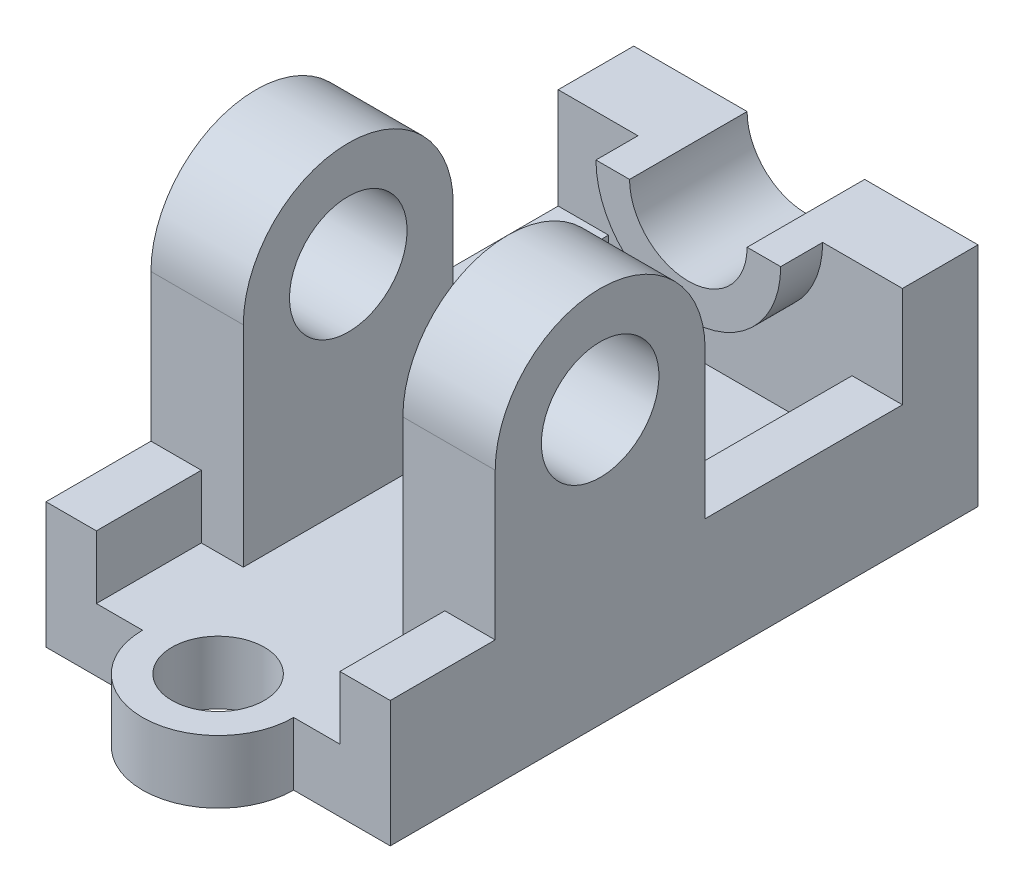
ISO-10303-21;
HEADER;
FILE_DESCRIPTION(('STEP AP214'),'2;1');
FILE_NAME('part.step','',(''),(''),'','','');
FILE_SCHEMA(('AUTOMOTIVE_DESIGN { 1 0 10303 214 1 1 1 1 }'));
ENDSEC;
DATA;
#1=APPLICATION_CONTEXT('core data for automotive mechanical design processes');
#2=APPLICATION_PROTOCOL_DEFINITION('international standard','automotive_design',2000,#1);
#3=PRODUCT_CONTEXT('',#1,'mechanical');
#4=PRODUCT('Part','Part','',(#3));
#5=PRODUCT_RELATED_PRODUCT_CATEGORY('part','',(#4));
#6=PRODUCT_DEFINITION_FORMATION('','',#4);
#7=PRODUCT_DEFINITION_CONTEXT('part definition',#1,'design');
#8=PRODUCT_DEFINITION('design','',#6,#7);
#9=PRODUCT_DEFINITION_SHAPE('','',#8);
#10=(LENGTH_UNIT() NAMED_UNIT(*) SI_UNIT(.MILLI.,.METRE.));
#11=(NAMED_UNIT(*) PLANE_ANGLE_UNIT() SI_UNIT($,.RADIAN.));
#12=(NAMED_UNIT(*) SI_UNIT($,.STERADIAN.) SOLID_ANGLE_UNIT());
#13=UNCERTAINTY_MEASURE_WITH_UNIT(LENGTH_MEASURE(1.E-05),#10,'distance_accuracy_value','');
#14=(GEOMETRIC_REPRESENTATION_CONTEXT(3) GLOBAL_UNCERTAINTY_ASSIGNED_CONTEXT((#13)) GLOBAL_UNIT_ASSIGNED_CONTEXT((#10,
#11,#12)) REPRESENTATION_CONTEXT('',''));
#15=CARTESIAN_POINT('',(0.,0.,0.));
#16=DIRECTION('',(0.,0.,1.));
#17=DIRECTION('',(1.,0.,0.));
#18=AXIS2_PLACEMENT_3D('',#15,#16,#17);
#19=CARTESIAN_POINT('',(41.,54.,-69.9999999999997));
#20=DIRECTION('',(0.,1.,0.));
#21=DIRECTION('',(0.,0.,1.));
#22=AXIS2_PLACEMENT_3D('',#19,#20,#21);
#23=PLANE('',#22);
#24=DIRECTION('',(0.,0.,-1.));
#25=VECTOR('',#24,1.);
#26=CARTESIAN_POINT('',(14.,54.,-26.));
#27=LINE('',#26,#25);
#28=CARTESIAN_POINT('',(14.,54.,-42.));
#29=VERTEX_POINT('',#28);
#30=CARTESIAN_POINT('',(14.,54.,-70.));
#31=VERTEX_POINT('',#30);
#32=EDGE_CURVE('E235',#29,#31,#27,.T.);
#33=ORIENTED_EDGE('',*,*,#32,.F.);
#34=DIRECTION('',(1.,0.,0.));
#35=VECTOR('',#34,1.);
#36=CARTESIAN_POINT('',(22.,54.,-42.));
#37=LINE('',#36,#35);
#38=CARTESIAN_POINT('',(22.,54.,-42.));
#39=VERTEX_POINT('',#38);
#40=EDGE_CURVE('E507',#29,#39,#37,.T.);
#41=ORIENTED_EDGE('',*,*,#40,.T.);
#42=DIRECTION('',(0.,0.,-1.));
#43=VECTOR('',#42,1.);
#44=CARTESIAN_POINT('',(22.,54.,-42.));
#45=LINE('',#44,#43);
#46=CARTESIAN_POINT('',(22.,54.,-51.9999999999998));
#47=VERTEX_POINT('',#46);
#48=EDGE_CURVE('E496',#39,#47,#45,.T.);
#49=ORIENTED_EDGE('',*,*,#48,.T.);
#50=DIRECTION('',(-1.,0.,0.));
#51=VECTOR('',#50,1.);
#52=CARTESIAN_POINT('',(40.9999999999999,54.,-51.9999999999997));
#53=LINE('',#52,#51);
#54=CARTESIAN_POINT('',(40.9999999999999,54.,-51.9999999999997));
#55=VERTEX_POINT('',#54);
#56=EDGE_CURVE('E70',#55,#47,#53,.T.);
#57=ORIENTED_EDGE('',*,*,#56,.F.);
#58=DIRECTION('',(0.,0.,-1.));
#59=VECTOR('',#58,1.);
#60=CARTESIAN_POINT('',(41.,54.,-69.9999999999997));
#61=LINE('',#60,#59);
#62=CARTESIAN_POINT('',(41.,54.,-69.9999999999997));
#63=VERTEX_POINT('',#62);
#64=EDGE_CURVE('E497',#55,#63,#61,.T.);
#65=ORIENTED_EDGE('',*,*,#64,.T.);
#66=DIRECTION('',(-1.,0.,0.));
#67=VECTOR('',#66,1.);
#68=CARTESIAN_POINT('',(41.,54.,-69.9999999999997));
#69=LINE('',#68,#67);
#70=EDGE_CURVE('E252',#63,#31,#69,.T.);
#71=ORIENTED_EDGE('',*,*,#70,.T.);
#72=EDGE_LOOP('',(#33,#41,#49,#57,#65,#71));
#73=FACE_BOUND('',#72,.T.);
#74=ADVANCED_FACE('F44',(#73),#23,.T.);
#75=CARTESIAN_POINT('',(0.,30.,0.));
#76=DIRECTION('',(0.,-1.,0.));
#77=DIRECTION('',(0.,0.,-1.));
#78=AXIS2_PLACEMENT_3D('',#75,#76,#77);
#79=PLANE('',#78);
#80=DIRECTION('',(0.,0.,-1.));
#81=VECTOR('',#80,1.);
#82=CARTESIAN_POINT('',(41.,30.,-70.));
#83=LINE('',#82,#81);
#84=CARTESIAN_POINT('',(41.,30.,-4.99999999999994));
#85=VERTEX_POINT('',#84);
#86=CARTESIAN_POINT('',(40.9999999999999,30.,-51.9999999999997));
#87=VERTEX_POINT('',#86);
#88=EDGE_CURVE('E342',#85,#87,#83,.T.);
#89=ORIENTED_EDGE('',*,*,#88,.T.);
#90=DIRECTION('',(-1.,0.,0.));
#91=VECTOR('',#90,1.);
#92=CARTESIAN_POINT('',(1.77833938051565E-13,30.,-51.9999999999999));
#93=LINE('',#92,#91);
#94=CARTESIAN_POINT('',(28.9999999999995,30.,-52.));
#95=VERTEX_POINT('',#94);
#96=EDGE_CURVE('E257',#87,#95,#93,.T.);
#97=ORIENTED_EDGE('',*,*,#96,.T.);
#98=DIRECTION('',(0.,0.,1.));
#99=VECTOR('',#98,1.);
#100=CARTESIAN_POINT('',(28.9999999999995,30.,70.));
#101=LINE('',#100,#99);
#102=CARTESIAN_POINT('',(28.9999999999995,30.,-4.99999999999992));
#103=VERTEX_POINT('',#102);
#104=EDGE_CURVE('E355',#95,#103,#101,.T.);
#105=ORIENTED_EDGE('',*,*,#104,.T.);
#106=DIRECTION('',(1.,0.,0.));
#107=VECTOR('',#106,1.);
#108=CARTESIAN_POINT('',(0.,30.,-4.99999999999994));
#109=LINE('',#108,#107);
#110=EDGE_CURVE('E294',#103,#85,#109,.T.);
#111=ORIENTED_EDGE('',*,*,#110,.T.);
#112=EDGE_LOOP('',(#89,#97,#105,#111));
#113=FACE_BOUND('',#112,.T.);
#114=ADVANCED_FACE('F532',(#113),#79,.F.);
#115=CARTESIAN_POINT('',(40.9999999999995,30.,70.));
#116=VERTEX_POINT('',#115);
#117=CARTESIAN_POINT('',(41.,30.,45.0000000000001));
#118=VERTEX_POINT('',#117);
#119=EDGE_CURVE('E344',#116,#118,#83,.T.);
#120=ORIENTED_EDGE('',*,*,#119,.T.);
#121=DIRECTION('',(-1.,0.,0.));
#122=VECTOR('',#121,1.);
#123=CARTESIAN_POINT('',(0.,30.,45.0000000000001));
#124=LINE('',#123,#122);
#125=CARTESIAN_POINT('',(28.9999999999995,30.,45.0000000000001));
#126=VERTEX_POINT('',#125);
#127=EDGE_CURVE('E304',#118,#126,#124,.T.);
#128=ORIENTED_EDGE('',*,*,#127,.T.);
#129=CARTESIAN_POINT('',(28.9999999999995,30.,70.));
#130=VERTEX_POINT('',#129);
#131=EDGE_CURVE('E353',#126,#130,#101,.T.);
#132=ORIENTED_EDGE('',*,*,#131,.T.);
#133=DIRECTION('',(1.,0.,0.));
#134=VECTOR('',#133,1.);
#135=CARTESIAN_POINT('',(40.9999999999995,30.,70.));
#136=LINE('',#135,#134);
#137=EDGE_CURVE('E356',#130,#116,#136,.T.);
#138=ORIENTED_EDGE('',*,*,#137,.T.);
#139=EDGE_LOOP('',(#120,#128,#132,#138));
#140=FACE_BOUND('',#139,.T.);
#141=ADVANCED_FACE('F538',(#140),#79,.F.);
#142=CARTESIAN_POINT('',(28.9999999999995,30.,70.));
#143=DIRECTION('',(1.,0.,0.));
#144=DIRECTION('',(0.,0.,-1.));
#145=AXIS2_PLACEMENT_3D('',#142,#143,#144);
#146=PLANE('',#145);
#147=ORIENTED_EDGE('',*,*,#131,.F.);
#148=DIRECTION('',(0.,-1.,0.));
#149=VECTOR('',#148,1.);
#150=CARTESIAN_POINT('',(28.9999999999995,30.,45.0000000000001));
#151=LINE('',#150,#149);
#152=CARTESIAN_POINT('',(28.9999999999995,15.,45.0000000000001));
#153=VERTEX_POINT('',#152);
#154=EDGE_CURVE('E53',#126,#153,#151,.T.);
#155=ORIENTED_EDGE('',*,*,#154,.T.);
#156=DIRECTION('',(0.,0.,1.));
#157=VECTOR('',#156,1.);
#158=CARTESIAN_POINT('',(28.9999999999995,15.,70.));
#159=LINE('',#158,#157);
#160=CARTESIAN_POINT('',(28.9999999999995,15.,70.));
#161=VERTEX_POINT('',#160);
#162=EDGE_CURVE('E368',#153,#161,#159,.T.);
#163=ORIENTED_EDGE('',*,*,#162,.T.);
#164=DIRECTION('',(0.,-1.,0.));
#165=VECTOR('',#164,1.);
#166=CARTESIAN_POINT('',(28.9999999999995,30.,70.));
#167=LINE('',#166,#165);
#168=EDGE_CURVE('E363',#130,#161,#167,.T.);
#169=ORIENTED_EDGE('',*,*,#168,.F.);
#170=EDGE_LOOP('',(#147,#155,#163,#169));
#171=FACE_BOUND('',#170,.T.);
#172=ADVANCED_FACE('F585',(#171),#146,.F.);
#173=CARTESIAN_POINT('',(-29.0000000000005,30.,-52.));
#174=DIRECTION('',(-1.,0.,0.));
#175=DIRECTION('',(0.,0.,1.));
#176=AXIS2_PLACEMENT_3D('',#173,#174,#175);
#177=PLANE('',#176);
#178=DIRECTION('',(0.,0.,-1.));
#179=VECTOR('',#178,1.);
#180=CARTESIAN_POINT('',(-29.0000000000005,30.,-52.));
#181=LINE('',#180,#179);
#182=CARTESIAN_POINT('',(-29.0000000000005,30.,-4.99999999999998));
#183=VERTEX_POINT('',#182);
#184=CARTESIAN_POINT('',(-29.0000000000005,30.,-52.));
#185=VERTEX_POINT('',#184);
#186=EDGE_CURVE('E347',#183,#185,#181,.T.);
#187=ORIENTED_EDGE('',*,*,#186,.F.);
#188=DIRECTION('',(0.,-1.,0.));
#189=VECTOR('',#188,1.);
#190=CARTESIAN_POINT('',(-29.0000000000005,30.,-4.99999999999996));
#191=LINE('',#190,#189);
#192=CARTESIAN_POINT('',(-29.0000000000005,15.,-5.00000000000002));
#193=VERTEX_POINT('',#192);
#194=EDGE_CURVE('E336',#183,#193,#191,.T.);
#195=ORIENTED_EDGE('',*,*,#194,.T.);
#196=DIRECTION('',(0.,0.,-1.));
#197=VECTOR('',#196,1.);
#198=CARTESIAN_POINT('',(-29.0000000000005,15.,-52.));
#199=LINE('',#198,#197);
#200=CARTESIAN_POINT('',(-29.0000000000005,15.,-52.));
#201=VERTEX_POINT('',#200);
#202=EDGE_CURVE('E338',#193,#201,#199,.T.);
#203=ORIENTED_EDGE('',*,*,#202,.T.);
#204=DIRECTION('',(0.,-1.,0.));
#205=VECTOR('',#204,1.);
#206=CARTESIAN_POINT('',(-29.0000000000005,30.,-52.));
#207=LINE('',#206,#205);
#208=EDGE_CURVE('E380',#185,#201,#207,.T.);
#209=ORIENTED_EDGE('',*,*,#208,.F.);
#210=EDGE_LOOP('',(#187,#195,#203,#209));
#211=FACE_BOUND('',#210,.T.);
#212=ADVANCED_FACE('F587',(#211),#177,.F.);
#213=ORIENTED_EDGE('',*,*,#186,.T.);
#214=CARTESIAN_POINT('',(-41.0000000000001,30.,-52.));
#215=VERTEX_POINT('',#214);
#216=EDGE_CURVE('E254',#185,#215,#93,.T.);
#217=ORIENTED_EDGE('',*,*,#216,.T.);
#218=DIRECTION('',(0.,0.,1.));
#219=VECTOR('',#218,1.);
#220=CARTESIAN_POINT('',(-41.0000000000005,30.,70.));
#221=LINE('',#220,#219);
#222=CARTESIAN_POINT('',(-41.0000000000002,30.,-5.));
#223=VERTEX_POINT('',#222);
#224=EDGE_CURVE('E349',#215,#223,#221,.T.);
#225=ORIENTED_EDGE('',*,*,#224,.T.);
#226=DIRECTION('',(1.,0.,0.));
#227=VECTOR('',#226,1.);
#228=CARTESIAN_POINT('',(0.,30.,-4.99999999999987));
#229=LINE('',#228,#227);
#230=EDGE_CURVE('E422',#223,#183,#229,.T.);
#231=ORIENTED_EDGE('',*,*,#230,.T.);
#232=EDGE_LOOP('',(#213,#217,#225,#231));
#233=FACE_BOUND('',#232,.T.);
#234=ADVANCED_FACE('F443',(#233),#79,.F.);
#235=CARTESIAN_POINT('',(41.,15.,0.));
#236=DIRECTION('',(-1.,0.,0.));
#237=DIRECTION('',(0.,0.,1.));
#238=AXIS2_PLACEMENT_3D('',#235,#236,#237);
#239=PLANE('',#238);
#240=CARTESIAN_POINT('',(41.,65.,20.0000000000003));
#241=DIRECTION('',(-1.,0.,0.));
#242=DIRECTION('',(0.,0.,1.));
#243=AXIS2_PLACEMENT_3D('',#240,#241,#242);
#244=CIRCLE('',#243,14.);
#245=CARTESIAN_POINT('',(41.,65.,34.0000000000003));
#246=VERTEX_POINT('',#245);
#247=EDGE_CURVE('E268',#246,#246,#244,.T.);
#248=ORIENTED_EDGE('',*,*,#247,.T.);
#249=EDGE_LOOP('',(#248));
#250=FACE_BOUND('',#249,.T.);
#251=DIRECTION('',(0.,0.,-1.));
#252=VECTOR('',#251,1.);
#253=CARTESIAN_POINT('',(41.,0.,0.));
#254=LINE('',#253,#252);
#255=CARTESIAN_POINT('',(40.9999999999995,0.,70.));
#256=VERTEX_POINT('',#255);
#257=CARTESIAN_POINT('',(41.,0.,-70.));
#258=VERTEX_POINT('',#257);
#259=EDGE_CURVE('E384',#256,#258,#254,.T.);
#260=ORIENTED_EDGE('',*,*,#259,.T.);
#261=DIRECTION('',(0.,-1.,0.));
#262=VECTOR('',#261,1.);
#263=CARTESIAN_POINT('',(41.,15.,-70.));
#264=LINE('',#263,#262);
#265=EDGE_CURVE('E416',#63,#258,#264,.T.);
#266=ORIENTED_EDGE('',*,*,#265,.F.);
#267=ORIENTED_EDGE('',*,*,#64,.F.);
#268=DIRECTION('',(0.,1.,0.));
#269=VECTOR('',#268,1.);
#270=CARTESIAN_POINT('',(40.9999999999999,30.,-51.9999999999997));
#271=LINE('',#270,#269);
#272=EDGE_CURVE('E492',#87,#55,#271,.T.);
#273=ORIENTED_EDGE('',*,*,#272,.F.);
#274=ORIENTED_EDGE('',*,*,#88,.F.);
#275=DIRECTION('',(0.,1.,0.));
#276=VECTOR('',#275,1.);
#277=CARTESIAN_POINT('',(41.,65.,-4.99999999999993));
#278=LINE('',#277,#276);
#279=CARTESIAN_POINT('',(41.,65.,-4.99999999999993));
#280=VERTEX_POINT('',#279);
#281=EDGE_CURVE('E275',#85,#280,#278,.T.);
#282=ORIENTED_EDGE('',*,*,#281,.T.);
#283=CARTESIAN_POINT('',(41.,65.,20.0000000000001));
#284=DIRECTION('',(1.,0.,0.));
#285=DIRECTION('',(0.,0.,-1.));
#286=AXIS2_PLACEMENT_3D('',#283,#284,#285);
#287=CIRCLE('',#286,25.);
#288=CARTESIAN_POINT('',(41.,65.,45.0000000000001));
#289=VERTEX_POINT('',#288);
#290=EDGE_CURVE('E289',#280,#289,#287,.T.);
#291=ORIENTED_EDGE('',*,*,#290,.T.);
#292=DIRECTION('',(0.,-1.,0.));
#293=VECTOR('',#292,1.);
#294=CARTESIAN_POINT('',(41.,65.,45.0000000000001));
#295=LINE('',#294,#293);
#296=EDGE_CURVE('E276',#289,#118,#295,.T.);
#297=ORIENTED_EDGE('',*,*,#296,.T.);
#298=ORIENTED_EDGE('',*,*,#119,.F.);
#299=DIRECTION('',(0.,-1.,0.));
#300=VECTOR('',#299,1.);
#301=CARTESIAN_POINT('',(40.9999999999995,15.,70.));
#302=LINE('',#301,#300);
#303=EDGE_CURVE('E391',#116,#256,#302,.T.);
#304=ORIENTED_EDGE('',*,*,#303,.T.);
#305=EDGE_LOOP('',(#260,#266,#267,#273,#274,#282,#291,#297,#298,#304));
#306=FACE_BOUND('',#305,.T.);
#307=ADVANCED_FACE('F50',(#250,#306),#239,.F.);
#308=CARTESIAN_POINT('',(41.,15.,-70.));
#309=DIRECTION('',(0.,0.,1.));
#310=DIRECTION('',(1.,0.,0.));
#311=AXIS2_PLACEMENT_3D('',#308,#309,#310);
#312=PLANE('',#311);
#313=CARTESIAN_POINT('',(-14.,54.,-70.));
#314=VERTEX_POINT('',#313);
#315=CARTESIAN_POINT('',(-41.,54.,-70.));
#316=VERTEX_POINT('',#315);
#317=EDGE_CURVE('E245',#314,#316,#69,.T.);
#318=ORIENTED_EDGE('',*,*,#317,.F.);
#319=CARTESIAN_POINT('',(0.,54.,-70.));
#320=DIRECTION('',(0.,0.,-1.));
#321=DIRECTION('',(-1.,0.,0.));
#322=AXIS2_PLACEMENT_3D('',#319,#320,#321);
#323=CIRCLE('',#322,14.);
#324=EDGE_CURVE('E230',#31,#314,#323,.T.);
#325=ORIENTED_EDGE('',*,*,#324,.F.);
#326=ORIENTED_EDGE('',*,*,#70,.F.);
#327=ORIENTED_EDGE('',*,*,#265,.T.);
#328=DIRECTION('',(-1.,0.,0.));
#329=VECTOR('',#328,1.);
#330=CARTESIAN_POINT('',(41.,0.,-70.));
#331=LINE('',#330,#329);
#332=CARTESIAN_POINT('',(-41.,0.,-70.));
#333=VERTEX_POINT('',#332);
#334=EDGE_CURVE('E393',#258,#333,#331,.T.);
#335=ORIENTED_EDGE('',*,*,#334,.T.);
#336=DIRECTION('',(0.,-1.,0.));
#337=VECTOR('',#336,1.);
#338=CARTESIAN_POINT('',(-41.,15.,-70.));
#339=LINE('',#338,#337);
#340=EDGE_CURVE('E248',#316,#333,#339,.T.);
#341=ORIENTED_EDGE('',*,*,#340,.F.);
#342=EDGE_LOOP('',(#318,#325,#326,#327,#335,#341));
#343=FACE_BOUND('',#342,.T.);
#344=ADVANCED_FACE('F250',(#343),#312,.F.);
#345=CARTESIAN_POINT('',(-41.,15.,-70.));
#346=DIRECTION('',(1.,0.,0.));
#347=DIRECTION('',(0.,0.,-1.));
#348=AXIS2_PLACEMENT_3D('',#345,#346,#347);
#349=PLANE('',#348);
#350=CARTESIAN_POINT('',(-41.0000000000003,65.,20.));
#351=DIRECTION('',(-1.,0.,0.));
#352=DIRECTION('',(0.,0.,1.));
#353=AXIS2_PLACEMENT_3D('',#350,#351,#352);
#354=CIRCLE('',#353,14.);
#355=CARTESIAN_POINT('',(-41.0000000000004,65.,34.));
#356=VERTEX_POINT('',#355);
#357=EDGE_CURVE('E261',#356,#356,#354,.T.);
#358=ORIENTED_EDGE('',*,*,#357,.F.);
#359=EDGE_LOOP('',(#358));
#360=FACE_BOUND('',#359,.T.);
#361=ORIENTED_EDGE('',*,*,#224,.F.);
#362=DIRECTION('',(0.,1.,0.));
#363=VECTOR('',#362,1.);
#364=CARTESIAN_POINT('',(-41.0000000000001,54.,-52.));
#365=LINE('',#364,#363);
#366=CARTESIAN_POINT('',(-41.0000000000001,54.,-52.));
#367=VERTEX_POINT('',#366);
#368=EDGE_CURVE('E486',#215,#367,#365,.T.);
#369=ORIENTED_EDGE('',*,*,#368,.T.);
#370=DIRECTION('',(0.,0.,-1.));
#371=VECTOR('',#370,1.);
#372=CARTESIAN_POINT('',(-41.,54.,-70.));
#373=LINE('',#372,#371);
#374=EDGE_CURVE('E256',#367,#316,#373,.T.);
#375=ORIENTED_EDGE('',*,*,#374,.T.);
#376=ORIENTED_EDGE('',*,*,#340,.T.);
#377=DIRECTION('',(0.,0.,1.));
#378=VECTOR('',#377,1.);
#379=CARTESIAN_POINT('',(-41.,0.,-70.));
#380=LINE('',#379,#378);
#381=CARTESIAN_POINT('',(-41.0000000000005,0.,70.));
#382=VERTEX_POINT('',#381);
#383=EDGE_CURVE('E396',#333,#382,#380,.T.);
#384=ORIENTED_EDGE('',*,*,#383,.T.);
#385=DIRECTION('',(0.,-1.,0.));
#386=VECTOR('',#385,1.);
#387=CARTESIAN_POINT('',(-41.0000000000005,15.,70.));
#388=LINE('',#387,#386);
#389=CARTESIAN_POINT('',(-41.0000000000005,30.,70.));
#390=VERTEX_POINT('',#389);
#391=EDGE_CURVE('E411',#390,#382,#388,.T.);
#392=ORIENTED_EDGE('',*,*,#391,.F.);
#393=CARTESIAN_POINT('',(-41.0000000000004,30.,45.));
#394=VERTEX_POINT('',#393);
#395=EDGE_CURVE('E343',#394,#390,#221,.T.);
#396=ORIENTED_EDGE('',*,*,#395,.F.);
#397=DIRECTION('',(0.,1.,0.));
#398=VECTOR('',#397,1.);
#399=CARTESIAN_POINT('',(-41.0000000000004,65.,45.));
#400=LINE('',#399,#398);
#401=CARTESIAN_POINT('',(-41.0000000000004,65.,45.));
#402=VERTEX_POINT('',#401);
#403=EDGE_CURVE('E308',#394,#402,#400,.T.);
#404=ORIENTED_EDGE('',*,*,#403,.T.);
#405=CARTESIAN_POINT('',(-41.0000000000003,65.,20.));
#406=DIRECTION('',(-1.,0.,0.));
#407=DIRECTION('',(0.,0.,1.));
#408=AXIS2_PLACEMENT_3D('',#405,#406,#407);
#409=CIRCLE('',#408,25.);
#410=CARTESIAN_POINT('',(-41.0000000000002,65.,-5.));
#411=VERTEX_POINT('',#410);
#412=EDGE_CURVE('E321',#402,#411,#409,.T.);
#413=ORIENTED_EDGE('',*,*,#412,.T.);
#414=DIRECTION('',(0.,-1.,0.));
#415=VECTOR('',#414,1.);
#416=CARTESIAN_POINT('',(-41.0000000000002,30.,-5.00000000000001));
#417=LINE('',#416,#415);
#418=EDGE_CURVE('E312',#411,#223,#417,.T.);
#419=ORIENTED_EDGE('',*,*,#418,.T.);
#420=EDGE_LOOP('',(#361,#369,#375,#376,#384,#392,#396,#404,#413,#419));
#421=FACE_BOUND('',#420,.T.);
#422=ADVANCED_FACE('F456',(#360,#421),#349,.F.);
#423=CARTESIAN_POINT('',(-41.0000000000005,15.,70.));
#424=DIRECTION('',(0.,0.,-1.));
#425=DIRECTION('',(-1.,0.,0.));
#426=AXIS2_PLACEMENT_3D('',#423,#424,#425);
#427=PLANE('',#426);
#428=DIRECTION('',(1.,0.,0.));
#429=VECTOR('',#428,1.);
#430=CARTESIAN_POINT('',(-41.0000000000005,0.,70.));
#431=LINE('',#430,#429);
#432=CARTESIAN_POINT('',(-18.0000000000005,0.,70.));
#433=VERTEX_POINT('',#432);
#434=EDGE_CURVE('E399',#382,#433,#431,.T.);
#435=ORIENTED_EDGE('',*,*,#434,.T.);
#436=DIRECTION('',(0.,-1.,0.));
#437=VECTOR('',#436,1.);
#438=CARTESIAN_POINT('',(-18.0000000000005,15.,70.));
#439=LINE('',#438,#437);
#440=CARTESIAN_POINT('',(-18.0000000000005,15.,70.));
#441=VERTEX_POINT('',#440);
#442=EDGE_CURVE('E408',#441,#433,#439,.T.);
#443=ORIENTED_EDGE('',*,*,#442,.F.);
#444=DIRECTION('',(1.,0.,0.));
#445=VECTOR('',#444,1.);
#446=CARTESIAN_POINT('',(-41.0000000000005,15.,70.));
#447=LINE('',#446,#445);
#448=CARTESIAN_POINT('',(-29.0000000000005,15.,70.));
#449=VERTEX_POINT('',#448);
#450=EDGE_CURVE('E381',#449,#441,#447,.T.);
#451=ORIENTED_EDGE('',*,*,#450,.F.);
#452=DIRECTION('',(0.,-1.,0.));
#453=VECTOR('',#452,1.);
#454=CARTESIAN_POINT('',(-29.0000000000005,30.,70.));
#455=LINE('',#454,#453);
#456=CARTESIAN_POINT('',(-29.0000000000005,30.,70.));
#457=VERTEX_POINT('',#456);
#458=EDGE_CURVE('E379',#457,#449,#455,.T.);
#459=ORIENTED_EDGE('',*,*,#458,.F.);
#460=DIRECTION('',(1.,0.,0.));
#461=VECTOR('',#460,1.);
#462=CARTESIAN_POINT('',(-41.0000000000005,30.,70.));
#463=LINE('',#462,#461);
#464=EDGE_CURVE('E350',#390,#457,#463,.T.);
#465=ORIENTED_EDGE('',*,*,#464,.F.);
#466=ORIENTED_EDGE('',*,*,#391,.T.);
#467=EDGE_LOOP('',(#435,#443,#451,#459,#465,#466));
#468=FACE_BOUND('',#467,.T.);
#469=ADVANCED_FACE('F457',(#468),#427,.F.);
#470=CARTESIAN_POINT('',(-4.85722573273506E-13,15.,70.));
#471=DIRECTION('',(0.,-1.,0.));
#472=DIRECTION('',(0.,0.,-1.));
#473=AXIS2_PLACEMENT_3D('',#470,#471,#472);
#474=CYLINDRICAL_SURFACE('',#473,18.);
#475=CARTESIAN_POINT('',(-4.85722573273506E-13,0.,70.));
#476=DIRECTION('',(0.,1.,0.));
#477=DIRECTION('',(0.,0.,1.));
#478=AXIS2_PLACEMENT_3D('',#475,#476,#477);
#479=CIRCLE('',#478,18.);
#480=CARTESIAN_POINT('',(17.9999999999995,0.,70.));
#481=VERTEX_POINT('',#480);
#482=EDGE_CURVE('E400',#433,#481,#479,.T.);
#483=ORIENTED_EDGE('',*,*,#482,.T.);
#484=DIRECTION('',(0.,-1.,0.));
#485=VECTOR('',#484,1.);
#486=CARTESIAN_POINT('',(17.9999999999995,15.,70.));
#487=LINE('',#486,#485);
#488=CARTESIAN_POINT('',(17.9999999999995,15.,70.));
#489=VERTEX_POINT('',#488);
#490=EDGE_CURVE('E409',#489,#481,#487,.T.);
#491=ORIENTED_EDGE('',*,*,#490,.F.);
#492=CARTESIAN_POINT('',(-4.85722573273506E-13,15.,70.));
#493=DIRECTION('',(0.,1.,0.));
#494=DIRECTION('',(0.,0.,1.));
#495=AXIS2_PLACEMENT_3D('',#492,#493,#494);
#496=CIRCLE('',#495,18.);
#497=EDGE_CURVE('E389',#441,#489,#496,.T.);
#498=ORIENTED_EDGE('',*,*,#497,.F.);
#499=ORIENTED_EDGE('',*,*,#442,.T.);
#500=EDGE_LOOP('',(#483,#491,#498,#499));
#501=FACE_BOUND('',#500,.T.);
#502=ADVANCED_FACE('F598',(#501),#474,.T.);
#503=CARTESIAN_POINT('',(17.9999999999995,15.,70.));
#504=DIRECTION('',(0.,0.,-1.));
#505=DIRECTION('',(-1.,0.,0.));
#506=AXIS2_PLACEMENT_3D('',#503,#504,#505);
#507=PLANE('',#506);
#508=DIRECTION('',(1.,0.,0.));
#509=VECTOR('',#508,1.);
#510=CARTESIAN_POINT('',(17.9999999999995,0.,70.));
#511=LINE('',#510,#509);
#512=EDGE_CURVE('E386',#481,#256,#511,.T.);
#513=ORIENTED_EDGE('',*,*,#512,.T.);
#514=ORIENTED_EDGE('',*,*,#303,.F.);
#515=ORIENTED_EDGE('',*,*,#137,.F.);
#516=ORIENTED_EDGE('',*,*,#168,.T.);
#517=DIRECTION('',(1.,0.,0.));
#518=VECTOR('',#517,1.);
#519=CARTESIAN_POINT('',(17.9999999999995,15.,70.));
#520=LINE('',#519,#518);
#521=EDGE_CURVE('E388',#489,#161,#520,.T.);
#522=ORIENTED_EDGE('',*,*,#521,.F.);
#523=ORIENTED_EDGE('',*,*,#490,.T.);
#524=EDGE_LOOP('',(#513,#514,#515,#516,#522,#523));
#525=FACE_BOUND('',#524,.T.);
#526=ADVANCED_FACE('F593',(#525),#507,.F.);
#527=CARTESIAN_POINT('',(-4.85722573273506E-13,15.,70.));
#528=DIRECTION('',(0.,1.,0.));
#529=DIRECTION('',(0.,0.,1.));
#530=AXIS2_PLACEMENT_3D('',#527,#528,#529);
#531=PLANE('',#530);
#532=CARTESIAN_POINT('',(-4.85722573273506E-13,15.,70.));
#533=DIRECTION('',(0.,1.,0.));
#534=DIRECTION('',(0.,0.,1.));
#535=AXIS2_PLACEMENT_3D('',#532,#533,#534);
#536=CIRCLE('',#535,11.);
#537=CARTESIAN_POINT('',(-4.85722573273506E-13,15.,81.));
#538=VERTEX_POINT('',#537);
#539=EDGE_CURVE('E514',#538,#538,#536,.T.);
#540=ORIENTED_EDGE('',*,*,#539,.F.);
#541=EDGE_LOOP('',(#540));
#542=FACE_BOUND('',#541,.T.);
#543=DIRECTION('',(1.,0.,0.));
#544=VECTOR('',#543,1.);
#545=CARTESIAN_POINT('',(19.,15.,45.0000000000001));
#546=LINE('',#545,#544);
#547=CARTESIAN_POINT('',(19.,15.,45.0000000000001));
#548=VERTEX_POINT('',#547);
#549=EDGE_CURVE('E291',#548,#153,#546,.T.);
#550=ORIENTED_EDGE('',*,*,#549,.F.);
#551=DIRECTION('',(0.,0.,-1.));
#552=VECTOR('',#551,1.);
#553=CARTESIAN_POINT('',(19.,15.,45.0000000000001));
#554=LINE('',#553,#552);
#555=CARTESIAN_POINT('',(19.,15.,-4.99999999999995));
#556=VERTEX_POINT('',#555);
#557=EDGE_CURVE('E271',#548,#556,#554,.T.);
#558=ORIENTED_EDGE('',*,*,#557,.T.);
#559=DIRECTION('',(1.,0.,0.));
#560=VECTOR('',#559,1.);
#561=CARTESIAN_POINT('',(19.,15.,-4.99999999999995));
#562=LINE('',#561,#560);
#563=CARTESIAN_POINT('',(28.9999999999995,15.,-4.99999999999995));
#564=VERTEX_POINT('',#563);
#565=EDGE_CURVE('E286',#556,#564,#562,.T.);
#566=ORIENTED_EDGE('',*,*,#565,.T.);
#567=CARTESIAN_POINT('',(28.9999999999995,15.,-52.));
#568=VERTEX_POINT('',#567);
#569=EDGE_CURVE('E367',#568,#564,#159,.T.);
#570=ORIENTED_EDGE('',*,*,#569,.F.);
#571=DIRECTION('',(1.,0.,0.));
#572=VECTOR('',#571,1.);
#573=CARTESIAN_POINT('',(28.9999999999995,15.,-52.));
#574=LINE('',#573,#572);
#575=EDGE_CURVE('E362',#201,#568,#574,.T.);
#576=ORIENTED_EDGE('',*,*,#575,.F.);
#577=ORIENTED_EDGE('',*,*,#202,.F.);
#578=DIRECTION('',(-1.,0.,0.));
#579=VECTOR('',#578,1.);
#580=CARTESIAN_POINT('',(-19.0000000000002,15.,-4.99999999999993));
#581=LINE('',#580,#579);
#582=CARTESIAN_POINT('',(-19.0000000000002,15.,-4.99999999999994));
#583=VERTEX_POINT('',#582);
#584=EDGE_CURVE('E318',#583,#193,#581,.T.);
#585=ORIENTED_EDGE('',*,*,#584,.F.);
#586=DIRECTION('',(0.,0.,1.));
#587=VECTOR('',#586,1.);
#588=CARTESIAN_POINT('',(-19.0000000000004,15.,45.0000000000001));
#589=LINE('',#588,#587);
#590=CARTESIAN_POINT('',(-19.0000000000004,15.,45.0000000000001));
#591=VERTEX_POINT('',#590);
#592=EDGE_CURVE('E315',#583,#591,#589,.T.);
#593=ORIENTED_EDGE('',*,*,#592,.T.);
#594=DIRECTION('',(-1.,0.,0.));
#595=VECTOR('',#594,1.);
#596=CARTESIAN_POINT('',(-19.0000000000004,15.,45.0000000000001));
#597=LINE('',#596,#595);
#598=CARTESIAN_POINT('',(-29.0000000000005,15.,45.0000000000001));
#599=VERTEX_POINT('',#598);
#600=EDGE_CURVE('E334',#591,#599,#597,.T.);
#601=ORIENTED_EDGE('',*,*,#600,.T.);
#602=EDGE_CURVE('E365',#449,#599,#199,.T.);
#603=ORIENTED_EDGE('',*,*,#602,.F.);
#604=ORIENTED_EDGE('',*,*,#450,.T.);
#605=ORIENTED_EDGE('',*,*,#497,.T.);
#606=ORIENTED_EDGE('',*,*,#521,.T.);
#607=ORIENTED_EDGE('',*,*,#162,.F.);
#608=EDGE_LOOP('',(#550,#558,#566,#570,#576,#577,#585,#593,#601,#603,#604,#605,#606,#607));
#609=FACE_BOUND('',#608,.T.);
#610=ADVANCED_FACE('F591',(#542,#609),#531,.T.);
#611=CARTESIAN_POINT('',(-4.85722573273506E-13,0.,70.));
#612=DIRECTION('',(0.,1.,0.));
#613=DIRECTION('',(0.,0.,1.));
#614=AXIS2_PLACEMENT_3D('',#611,#612,#613);
#615=PLANE('',#614);
#616=CARTESIAN_POINT('',(-4.85722573273506E-13,0.,70.));
#617=DIRECTION('',(0.,1.,0.));
#618=DIRECTION('',(0.,0.,1.));
#619=AXIS2_PLACEMENT_3D('',#616,#617,#618);
#620=CIRCLE('',#619,11.);
#621=CARTESIAN_POINT('',(-4.85722573273506E-13,0.,81.));
#622=VERTEX_POINT('',#621);
#623=EDGE_CURVE('E47',#622,#622,#620,.T.);
#624=ORIENTED_EDGE('',*,*,#623,.T.);
#625=EDGE_LOOP('',(#624));
#626=FACE_BOUND('',#625,.T.);
#627=ORIENTED_EDGE('',*,*,#434,.F.);
#628=ORIENTED_EDGE('',*,*,#383,.F.);
#629=ORIENTED_EDGE('',*,*,#334,.F.);
#630=ORIENTED_EDGE('',*,*,#259,.F.);
#631=ORIENTED_EDGE('',*,*,#512,.F.);
#632=ORIENTED_EDGE('',*,*,#482,.F.);
#633=EDGE_LOOP('',(#627,#628,#629,#630,#631,#632));
#634=FACE_BOUND('',#633,.T.);
#635=ADVANCED_FACE('F455',(#626,#634),#615,.F.);
#636=ORIENTED_EDGE('',*,*,#602,.T.);
#637=DIRECTION('',(0.,1.,0.));
#638=VECTOR('',#637,1.);
#639=CARTESIAN_POINT('',(-29.0000000000005,30.,45.0000000000001));
#640=LINE('',#639,#638);
#641=CARTESIAN_POINT('',(-29.0000000000005,30.,45.));
#642=VERTEX_POINT('',#641);
#643=EDGE_CURVE('E328',#599,#642,#640,.T.);
#644=ORIENTED_EDGE('',*,*,#643,.T.);
#645=EDGE_CURVE('E351',#457,#642,#181,.T.);
#646=ORIENTED_EDGE('',*,*,#645,.F.);
#647=ORIENTED_EDGE('',*,*,#458,.T.);
#648=EDGE_LOOP('',(#636,#644,#646,#647));
#649=FACE_BOUND('',#648,.T.);
#650=ADVANCED_FACE('F589',(#649),#177,.F.);
#651=CARTESIAN_POINT('',(28.9999999999995,30.,-52.));
#652=DIRECTION('',(0.,0.,-1.));
#653=DIRECTION('',(-1.,0.,0.));
#654=AXIS2_PLACEMENT_3D('',#651,#652,#653);
#655=PLANE('',#654);
#656=ORIENTED_EDGE('',*,*,#56,.T.);
#657=CARTESIAN_POINT('',(0.,54.,-52.));
#658=DIRECTION('',(0.,0.,-1.));
#659=DIRECTION('',(-1.,0.,0.));
#660=AXIS2_PLACEMENT_3D('',#657,#658,#659);
#661=CIRCLE('',#660,22.);
#662=CARTESIAN_POINT('',(-22.,54.,-51.9999999999997));
#663=VERTEX_POINT('',#662);
#664=EDGE_CURVE('E494',#47,#663,#661,.T.);
#665=ORIENTED_EDGE('',*,*,#664,.T.);
#666=EDGE_CURVE('E251',#663,#367,#53,.T.);
#667=ORIENTED_EDGE('',*,*,#666,.T.);
#668=ORIENTED_EDGE('',*,*,#368,.F.);
#669=ORIENTED_EDGE('',*,*,#216,.F.);
#670=ORIENTED_EDGE('',*,*,#208,.T.);
#671=ORIENTED_EDGE('',*,*,#575,.T.);
#672=DIRECTION('',(0.,-1.,0.));
#673=VECTOR('',#672,1.);
#674=CARTESIAN_POINT('',(28.9999999999995,30.,-52.));
#675=LINE('',#674,#673);
#676=EDGE_CURVE('E372',#95,#568,#675,.T.);
#677=ORIENTED_EDGE('',*,*,#676,.F.);
#678=ORIENTED_EDGE('',*,*,#96,.F.);
#679=ORIENTED_EDGE('',*,*,#272,.T.);
#680=EDGE_LOOP('',(#656,#665,#667,#668,#669,#670,#671,#677,#678,#679));
#681=FACE_BOUND('',#680,.T.);
#682=ADVANCED_FACE('F491',(#681),#655,.F.);
#683=ORIENTED_EDGE('',*,*,#569,.T.);
#684=DIRECTION('',(0.,1.,0.));
#685=VECTOR('',#684,1.);
#686=CARTESIAN_POINT('',(28.9999999999995,30.,-4.99999999999995));
#687=LINE('',#686,#685);
#688=EDGE_CURVE('E425',#564,#103,#687,.T.);
#689=ORIENTED_EDGE('',*,*,#688,.T.);
#690=ORIENTED_EDGE('',*,*,#104,.F.);
#691=ORIENTED_EDGE('',*,*,#676,.T.);
#692=EDGE_LOOP('',(#683,#689,#690,#691));
#693=FACE_BOUND('',#692,.T.);
#694=ADVANCED_FACE('F576',(#693),#146,.F.);
#695=ORIENTED_EDGE('',*,*,#645,.T.);
#696=DIRECTION('',(-1.,0.,0.));
#697=VECTOR('',#696,1.);
#698=CARTESIAN_POINT('',(-1.53894754083086E-13,30.,45.0000000000001));
#699=LINE('',#698,#697);
#700=EDGE_CURVE('E418',#642,#394,#699,.T.);
#701=ORIENTED_EDGE('',*,*,#700,.T.);
#702=ORIENTED_EDGE('',*,*,#395,.T.);
#703=ORIENTED_EDGE('',*,*,#464,.T.);
#704=EDGE_LOOP('',(#695,#701,#702,#703));
#705=FACE_BOUND('',#704,.T.);
#706=ADVANCED_FACE('F467',(#705),#79,.F.);
#707=CARTESIAN_POINT('',(-19.0000000000002,30.,-4.99999999999993));
#708=DIRECTION('',(0.,0.,-1.));
#709=DIRECTION('',(-1.,0.,0.));
#710=AXIS2_PLACEMENT_3D('',#707,#708,#709);
#711=PLANE('',#710);
#712=ORIENTED_EDGE('',*,*,#194,.F.);
#713=ORIENTED_EDGE('',*,*,#230,.F.);
#714=ORIENTED_EDGE('',*,*,#418,.F.);
#715=DIRECTION('',(-1.,0.,0.));
#716=VECTOR('',#715,1.);
#717=CARTESIAN_POINT('',(-19.0000000000002,65.,-4.99999999999993));
#718=LINE('',#717,#716);
#719=CARTESIAN_POINT('',(-19.0000000000002,65.,-4.99999999999993));
#720=VERTEX_POINT('',#719);
#721=EDGE_CURVE('E326',#720,#411,#718,.T.);
#722=ORIENTED_EDGE('',*,*,#721,.F.);
#723=DIRECTION('',(0.,-1.,0.));
#724=VECTOR('',#723,1.);
#725=CARTESIAN_POINT('',(-19.0000000000002,15.,-4.99999999999993));
#726=LINE('',#725,#724);
#727=EDGE_CURVE('E307',#720,#583,#726,.T.);
#728=ORIENTED_EDGE('',*,*,#727,.T.);
#729=ORIENTED_EDGE('',*,*,#584,.T.);
#730=EDGE_LOOP('',(#712,#713,#714,#722,#728,#729));
#731=FACE_BOUND('',#730,.T.);
#732=ADVANCED_FACE('F484',(#731),#711,.T.);
#733=CARTESIAN_POINT('',(-19.0000000000004,65.,45.0000000000001));
#734=DIRECTION('',(0.,0.,1.));
#735=DIRECTION('',(1.,0.,0.));
#736=AXIS2_PLACEMENT_3D('',#733,#734,#735);
#737=PLANE('',#736);
#738=ORIENTED_EDGE('',*,*,#643,.F.);
#739=ORIENTED_EDGE('',*,*,#600,.F.);
#740=DIRECTION('',(0.,1.,0.));
#741=VECTOR('',#740,1.);
#742=CARTESIAN_POINT('',(-19.0000000000004,30.,45.0000000000001));
#743=LINE('',#742,#741);
#744=CARTESIAN_POINT('',(-19.0000000000004,65.,45.0000000000001));
#745=VERTEX_POINT('',#744);
#746=EDGE_CURVE('E314',#591,#745,#743,.T.);
#747=ORIENTED_EDGE('',*,*,#746,.T.);
#748=DIRECTION('',(-1.,0.,0.));
#749=VECTOR('',#748,1.);
#750=CARTESIAN_POINT('',(-19.0000000000004,65.,45.0000000000001));
#751=LINE('',#750,#749);
#752=EDGE_CURVE('E327',#745,#402,#751,.T.);
#753=ORIENTED_EDGE('',*,*,#752,.T.);
#754=ORIENTED_EDGE('',*,*,#403,.F.);
#755=ORIENTED_EDGE('',*,*,#700,.F.);
#756=EDGE_LOOP('',(#738,#739,#747,#753,#754,#755));
#757=FACE_BOUND('',#756,.T.);
#758=ADVANCED_FACE('F473',(#757),#737,.T.);
#759=CARTESIAN_POINT('',(-19.0000000000003,65.,20.0000000000001));
#760=DIRECTION('',(-1.,0.,0.));
#761=DIRECTION('',(0.,0.,1.));
#762=AXIS2_PLACEMENT_3D('',#759,#760,#761);
#763=CYLINDRICAL_SURFACE('',#762,25.);
#764=ORIENTED_EDGE('',*,*,#412,.F.);
#765=ORIENTED_EDGE('',*,*,#752,.F.);
#766=CARTESIAN_POINT('',(-19.0000000000003,65.,20.0000000000001));
#767=DIRECTION('',(-1.,0.,0.));
#768=DIRECTION('',(0.,0.,1.));
#769=AXIS2_PLACEMENT_3D('',#766,#767,#768);
#770=CIRCLE('',#769,25.);
#771=EDGE_CURVE('E320',#745,#720,#770,.T.);
#772=ORIENTED_EDGE('',*,*,#771,.T.);
#773=ORIENTED_EDGE('',*,*,#721,.T.);
#774=EDGE_LOOP('',(#764,#765,#772,#773));
#775=FACE_BOUND('',#774,.T.);
#776=ADVANCED_FACE('F478',(#775),#763,.T.);
#777=CARTESIAN_POINT('',(-19.0000000000003,65.,20.0000000000001));
#778=DIRECTION('',(-1.,0.,0.));
#779=DIRECTION('',(0.,0.,1.));
#780=AXIS2_PLACEMENT_3D('',#777,#778,#779);
#781=PLANE('',#780);
#782=CARTESIAN_POINT('',(-19.0000000000003,65.,20.0000000000001));
#783=DIRECTION('',(-1.,0.,0.));
#784=DIRECTION('',(0.,0.,1.));
#785=AXIS2_PLACEMENT_3D('',#782,#783,#784);
#786=CIRCLE('',#785,14.);
#787=CARTESIAN_POINT('',(-19.0000000000004,65.,34.0000000000001));
#788=VERTEX_POINT('',#787);
#789=EDGE_CURVE('E266',#788,#788,#786,.T.);
#790=ORIENTED_EDGE('',*,*,#789,.T.);
#791=EDGE_LOOP('',(#790));
#792=FACE_BOUND('',#791,.T.);
#793=ORIENTED_EDGE('',*,*,#727,.F.);
#794=ORIENTED_EDGE('',*,*,#771,.F.);
#795=ORIENTED_EDGE('',*,*,#746,.F.);
#796=ORIENTED_EDGE('',*,*,#592,.F.);
#797=EDGE_LOOP('',(#793,#794,#795,#796));
#798=FACE_BOUND('',#797,.T.);
#799=ADVANCED_FACE('F561',(#792,#798),#781,.F.);
#800=CARTESIAN_POINT('',(19.,65.,45.0000000000001));
#801=DIRECTION('',(0.,0.,1.));
#802=DIRECTION('',(1.,0.,0.));
#803=AXIS2_PLACEMENT_3D('',#800,#801,#802);
#804=PLANE('',#803);
#805=ORIENTED_EDGE('',*,*,#127,.F.);
#806=ORIENTED_EDGE('',*,*,#296,.F.);
#807=DIRECTION('',(1.,0.,0.));
#808=VECTOR('',#807,1.);
#809=CARTESIAN_POINT('',(19.,65.,45.0000000000001));
#810=LINE('',#809,#808);
#811=CARTESIAN_POINT('',(19.,65.,45.0000000000001));
#812=VERTEX_POINT('',#811);
#813=EDGE_CURVE('E298',#812,#289,#810,.T.);
#814=ORIENTED_EDGE('',*,*,#813,.F.);
#815=DIRECTION('',(0.,-1.,0.));
#816=VECTOR('',#815,1.);
#817=CARTESIAN_POINT('',(19.,65.,45.0000000000001));
#818=LINE('',#817,#816);
#819=EDGE_CURVE('E285',#812,#548,#818,.T.);
#820=ORIENTED_EDGE('',*,*,#819,.T.);
#821=ORIENTED_EDGE('',*,*,#549,.T.);
#822=ORIENTED_EDGE('',*,*,#154,.F.);
#823=EDGE_LOOP('',(#805,#806,#814,#820,#821,#822));
#824=FACE_BOUND('',#823,.T.);
#825=ADVANCED_FACE('F560',(#824),#804,.T.);
#826=CARTESIAN_POINT('',(19.,65.,-4.99999999999993));
#827=DIRECTION('',(0.,0.,-1.));
#828=DIRECTION('',(0.,1.,0.));
#829=AXIS2_PLACEMENT_3D('',#826,#827,#828);
#830=PLANE('',#829);
#831=ORIENTED_EDGE('',*,*,#110,.F.);
#832=ORIENTED_EDGE('',*,*,#688,.F.);
#833=ORIENTED_EDGE('',*,*,#565,.F.);
#834=DIRECTION('',(0.,1.,0.));
#835=VECTOR('',#834,1.);
#836=CARTESIAN_POINT('',(19.,65.,-4.99999999999993));
#837=LINE('',#836,#835);
#838=CARTESIAN_POINT('',(19.,65.,-4.99999999999993));
#839=VERTEX_POINT('',#838);
#840=EDGE_CURVE('E279',#556,#839,#837,.T.);
#841=ORIENTED_EDGE('',*,*,#840,.T.);
#842=DIRECTION('',(1.,0.,0.));
#843=VECTOR('',#842,1.);
#844=CARTESIAN_POINT('',(19.,65.,-4.99999999999993));
#845=LINE('',#844,#843);
#846=EDGE_CURVE('E296',#839,#280,#845,.T.);
#847=ORIENTED_EDGE('',*,*,#846,.T.);
#848=ORIENTED_EDGE('',*,*,#281,.F.);
#849=EDGE_LOOP('',(#831,#832,#833,#841,#847,#848));
#850=FACE_BOUND('',#849,.T.);
#851=ADVANCED_FACE('F557',(#850),#830,.T.);
#852=CARTESIAN_POINT('',(19.,65.,20.0000000000001));
#853=DIRECTION('',(1.,0.,0.));
#854=DIRECTION('',(0.,0.,-1.));
#855=AXIS2_PLACEMENT_3D('',#852,#853,#854);
#856=CYLINDRICAL_SURFACE('',#855,25.);
#857=ORIENTED_EDGE('',*,*,#290,.F.);
#858=ORIENTED_EDGE('',*,*,#846,.F.);
#859=CARTESIAN_POINT('',(19.,65.,20.0000000000001));
#860=DIRECTION('',(1.,0.,0.));
#861=DIRECTION('',(0.,0.,-1.));
#862=AXIS2_PLACEMENT_3D('',#859,#860,#861);
#863=CIRCLE('',#862,25.);
#864=EDGE_CURVE('E277',#839,#812,#863,.T.);
#865=ORIENTED_EDGE('',*,*,#864,.T.);
#866=ORIENTED_EDGE('',*,*,#813,.T.);
#867=EDGE_LOOP('',(#857,#858,#865,#866));
#868=FACE_BOUND('',#867,.T.);
#869=ADVANCED_FACE('F558',(#868),#856,.T.);
#870=CARTESIAN_POINT('',(19.,65.,20.0000000000001));
#871=DIRECTION('',(1.,0.,0.));
#872=DIRECTION('',(0.,0.,-1.));
#873=AXIS2_PLACEMENT_3D('',#870,#871,#872);
#874=PLANE('',#873);
#875=CARTESIAN_POINT('',(19.,65.,20.0000000000002));
#876=DIRECTION('',(1.,0.,0.));
#877=DIRECTION('',(0.,0.,-1.));
#878=AXIS2_PLACEMENT_3D('',#875,#876,#877);
#879=CIRCLE('',#878,14.);
#880=CARTESIAN_POINT('',(19.,65.,6.00000000000021));
#881=VERTEX_POINT('',#880);
#882=EDGE_CURVE('E262',#881,#881,#879,.T.);
#883=ORIENTED_EDGE('',*,*,#882,.T.);
#884=EDGE_LOOP('',(#883));
#885=FACE_BOUND('',#884,.T.);
#886=ORIENTED_EDGE('',*,*,#557,.F.);
#887=ORIENTED_EDGE('',*,*,#819,.F.);
#888=ORIENTED_EDGE('',*,*,#864,.F.);
#889=ORIENTED_EDGE('',*,*,#840,.F.);
#890=EDGE_LOOP('',(#886,#887,#888,#889));
#891=FACE_BOUND('',#890,.T.);
#892=ADVANCED_FACE('F435',(#885,#891),#874,.F.);
#893=CARTESIAN_POINT('',(64.9999999999997,65.,20.0000000000004));
#894=DIRECTION('',(-1.,0.,0.));
#895=DIRECTION('',(0.,0.,1.));
#896=AXIS2_PLACEMENT_3D('',#893,#894,#895);
#897=CYLINDRICAL_SURFACE('',#896,14.);
#898=ORIENTED_EDGE('',*,*,#882,.F.);
#899=EDGE_LOOP('',(#898));
#900=FACE_BOUND('',#899,.T.);
#901=ORIENTED_EDGE('',*,*,#247,.F.);
#902=EDGE_LOOP('',(#901));
#903=FACE_BOUND('',#902,.T.);
#904=ADVANCED_FACE('F434',(#900,#903),#897,.F.);
#905=ORIENTED_EDGE('',*,*,#357,.T.);
#906=EDGE_LOOP('',(#905));
#907=FACE_BOUND('',#906,.T.);
#908=ORIENTED_EDGE('',*,*,#789,.F.);
#909=EDGE_LOOP('',(#908));
#910=FACE_BOUND('',#909,.T.);
#911=ADVANCED_FACE('F438',(#907,#910),#897,.F.);
#912=DIRECTION('',(0.,0.,-1.));
#913=VECTOR('',#912,1.);
#914=CARTESIAN_POINT('',(-14.,54.,-26.));
#915=LINE('',#914,#913);
#916=CARTESIAN_POINT('',(-14.,54.,-42.));
#917=VERTEX_POINT('',#916);
#918=EDGE_CURVE('E64',#917,#314,#915,.T.);
#919=ORIENTED_EDGE('',*,*,#918,.T.);
#920=ORIENTED_EDGE('',*,*,#317,.T.);
#921=ORIENTED_EDGE('',*,*,#374,.F.);
#922=ORIENTED_EDGE('',*,*,#666,.F.);
#923=DIRECTION('',(0.,0.,-1.));
#924=VECTOR('',#923,1.);
#925=CARTESIAN_POINT('',(-22.,54.,-42.));
#926=LINE('',#925,#924);
#927=CARTESIAN_POINT('',(-22.,54.,-42.));
#928=VERTEX_POINT('',#927);
#929=EDGE_CURVE('E505',#928,#663,#926,.T.);
#930=ORIENTED_EDGE('',*,*,#929,.F.);
#931=EDGE_CURVE('E244',#928,#917,#37,.T.);
#932=ORIENTED_EDGE('',*,*,#931,.T.);
#933=EDGE_LOOP('',(#919,#920,#921,#922,#930,#932));
#934=FACE_BOUND('',#933,.T.);
#935=ADVANCED_FACE('F239',(#934),#23,.T.);
#936=CARTESIAN_POINT('',(0.,54.,-42.));
#937=DIRECTION('',(0.,0.,-1.));
#938=DIRECTION('',(-1.,0.,0.));
#939=AXIS2_PLACEMENT_3D('',#936,#937,#938);
#940=CYLINDRICAL_SURFACE('',#939,22.);
#941=ORIENTED_EDGE('',*,*,#664,.F.);
#942=ORIENTED_EDGE('',*,*,#48,.F.);
#943=CARTESIAN_POINT('',(0.,54.,-42.));
#944=DIRECTION('',(0.,0.,-1.));
#945=DIRECTION('',(-1.,0.,0.));
#946=AXIS2_PLACEMENT_3D('',#943,#944,#945);
#947=CIRCLE('',#946,22.);
#948=EDGE_CURVE('E508',#39,#928,#947,.T.);
#949=ORIENTED_EDGE('',*,*,#948,.T.);
#950=ORIENTED_EDGE('',*,*,#929,.T.);
#951=EDGE_LOOP('',(#941,#942,#949,#950));
#952=FACE_BOUND('',#951,.T.);
#953=ADVANCED_FACE('F543',(#952),#940,.T.);
#954=CARTESIAN_POINT('',(0.,54.,-42.));
#955=DIRECTION('',(0.,0.,-1.));
#956=DIRECTION('',(-1.,0.,0.));
#957=AXIS2_PLACEMENT_3D('',#954,#955,#956);
#958=PLANE('',#957);
#959=ORIENTED_EDGE('',*,*,#40,.F.);
#960=CARTESIAN_POINT('',(0.,54.,-42.));
#961=DIRECTION('',(0.,0.,-1.));
#962=DIRECTION('',(-1.,0.,0.));
#963=AXIS2_PLACEMENT_3D('',#960,#961,#962);
#964=CIRCLE('',#963,14.);
#965=EDGE_CURVE('E11',#29,#917,#964,.T.);
#966=ORIENTED_EDGE('',*,*,#965,.T.);
#967=ORIENTED_EDGE('',*,*,#931,.F.);
#968=ORIENTED_EDGE('',*,*,#948,.F.);
#969=EDGE_LOOP('',(#959,#966,#967,#968));
#970=FACE_BOUND('',#969,.T.);
#971=ADVANCED_FACE('F529',(#970),#958,.F.);
#972=CARTESIAN_POINT('',(0.,54.,-26.));
#973=DIRECTION('',(0.,0.,-1.));
#974=DIRECTION('',(-1.,0.,0.));
#975=AXIS2_PLACEMENT_3D('',#972,#973,#974);
#976=CYLINDRICAL_SURFACE('',#975,14.);
#977=ORIENTED_EDGE('',*,*,#32,.T.);
#978=ORIENTED_EDGE('',*,*,#324,.T.);
#979=ORIENTED_EDGE('',*,*,#918,.F.);
#980=ORIENTED_EDGE('',*,*,#965,.F.);
#981=EDGE_LOOP('',(#977,#978,#979,#980));
#982=FACE_BOUND('',#981,.T.);
#983=ADVANCED_FACE('F229',(#982),#976,.F.);
#984=CARTESIAN_POINT('',(-4.85722573273506E-13,-29.,70.));
#985=DIRECTION('',(0.,1.,0.));
#986=DIRECTION('',(0.,0.,1.));
#987=AXIS2_PLACEMENT_3D('',#984,#985,#986);
#988=CYLINDRICAL_SURFACE('',#987,11.);
#989=ORIENTED_EDGE('',*,*,#539,.T.);
#990=EDGE_LOOP('',(#989));
#991=FACE_BOUND('',#990,.T.);
#992=ORIENTED_EDGE('',*,*,#623,.F.);
#993=EDGE_LOOP('',(#992));
#994=FACE_BOUND('',#993,.T.);
#995=ADVANCED_FACE('F524',(#991,#994),#988,.F.);
#996=CLOSED_SHELL('',(#74,#114,#141,#172,#212,#234,#307,#344,#422,#469,#502,#526,#610,#635,#650,
#682,#694,#706,#732,#758,#776,#799,#825,#851,#869,#892,#904,#911,#935,#953,#971,#983,#995));
#997=MANIFOLD_SOLID_BREP('B2',#996);
#998=ADVANCED_BREP_SHAPE_REPRESENTATION('',(#18,#997),#14);
#999=SHAPE_DEFINITION_REPRESENTATION(#9,#998);
ENDSEC;
END-ISO-10303-21;
